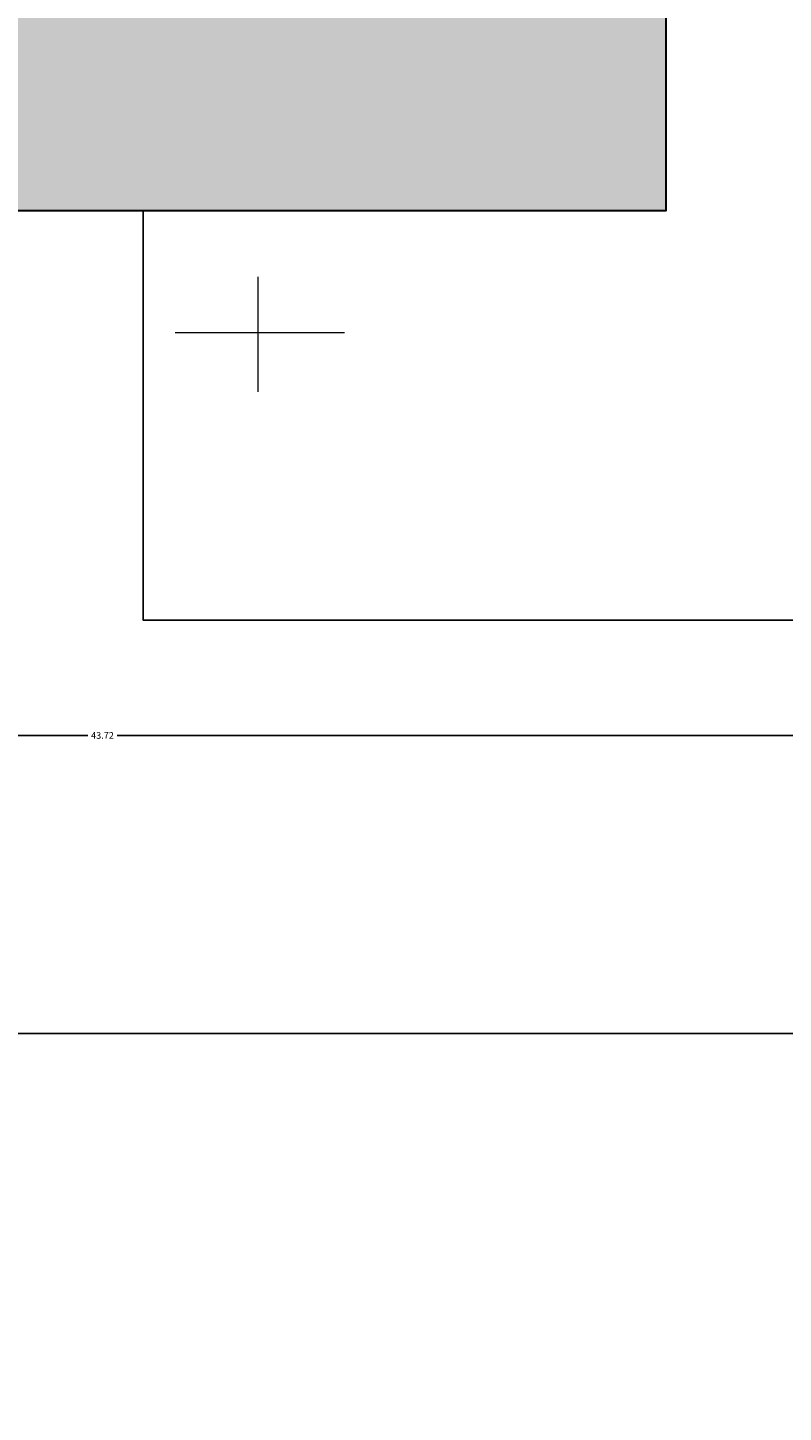
# Model space of a CAD drawing. Units: millimetres. Extents: x -8 to 285, y 5 to 221.
# Tile 12 of 30: x 27 to 47, y 113 to 150. Entities that reach past the tile are written whole.
import ezdxf

# ---------------------------------------------------------------- set-up
doc = ezdxf.new("R2010")
doc.units = ezdxf.units.MM
for name, color, linetype, lineweight in [('A-ANNO-DIMS', 2, 'Continuous', 18), ('E-ANNO-SYMB', 7, 'Continuous', 18), ('E-EQPM-PATT', 252, 'Continuous', 13), ('E-POWR-DC-LINK', 4, 'Continuous', 25), ('E-POWR-PV', 7, 'Continuous', 30)]:
    doc.layers.add(name, color=color, linetype=linetype, lineweight=lineweight)
doc.layers.add('E-POWR-DC-POS', color=30, linetype='Continuous', lineweight=25, true_color=0xf26722)
doc.styles.get("Standard").update_dxf_attribs({"font": 'arial.ttf'})
doc.dimstyles.get("Standard").update_dxf_attribs({"dimtxt": 0.18, "dimasz": 0.18, "dimexe": 0.18, "dimexo": 0.0625, "dimgap": 0.09, "dimtad": 0, "dimtih": 1, "dimtoh": 1, "dimdec": 4, "dimzin": 0, "dimdsep": 46, "dimtxsty": 'Standard', "dimcen": 0.09, "dimadec": 0, "dimazin": 0, "dimtfac": 1, "dimtdec": 4, "dimtofl": 0, "dimtmove": 0, "dimatfit": 3, "dimfxl": 1, "dimtolj": 1, "dimtzin": 0, "dimarcsym": 0})

# ---------------------------------------------------------------- blocks, each defined once
blk = doc.blocks.new('PV-MODULE-12V')
blk.add_lwpolyline([(0, 47), (37, 47), (37, 0), (0, 0)], close=True)
blk = doc.blocks.new('POLARITY-POSITIVE')
for p, q in [((2.22, 3.095), (2.22, 0)), ((0, 1.599), (4.543, 1.599))]:
    blk.add_line(p, q)
blk = doc.blocks.new('*D9')
at = {"layer": 'A-ANNO-DIMS', "color": 0, "lineweight": -2, "transparency": 16777216}
for p, q in [((6.672, 133.79), (6.672, 220.737)), ((270.919, 206.519), (270.919, 220.737)), ((6.852, 220.557), (138.33, 220.557)), ((270.739, 220.557), (139.262, 220.557))]:
    blk.add_line(p, q, dxfattribs=at)
at = {"layer": 'A-ANNO-DIMS', "color": 0, "transparency": 16777216}
for points in [[(6.852, 220.587), (6.852, 220.527), (6.672, 220.557)], [(270.739, 220.587), (270.739, 220.527), (270.919, 220.557)]]:
    blk.add_solid(points, dxfattribs=at)
at = {"layer": 'Defpoints', "color": 0, "transparency": 16777216}
for p in [(270.919, 220.557), (270.919, 206.457), (6.672, 133.727)]:
    blk.add_point(p, dxfattribs=at)
at = {"layer": 'A-ANNO-DIMS', "color": 0, "transparency": 16777216, "insert": (138.796, 220.557), "char_height": 0.18, "attachment_point": 5}
blk.add_mtext('\\A1;264.25', dxfattribs=at)
blk = doc.blocks.new('*D10')
at = {"layer": 'A-ANNO-DIMS', "color": 0, "lineweight": -2, "transparency": 16777216}
for p, q in [((145.103, 206.457), (-7.608, 206.457)), ((-7.428, 206.277), (-7.428, 113.161)), ((-7.428, 19.682), (-7.428, 112.797)), ((30.453, 19.502), (-7.608, 19.502))]:
    blk.add_line(p, q, dxfattribs=at)
at = {"layer": 'A-ANNO-DIMS', "color": 0, "transparency": 16777216}
for points in [[(-7.458, 206.277), (-7.398, 206.277), (-7.428, 206.457)], [(-7.458, 19.682), (-7.398, 19.682), (-7.428, 19.502)]]:
    blk.add_solid(points, dxfattribs=at)
at = {"layer": 'Defpoints', "color": 0, "transparency": 16777216}
for p in [(-7.428, 206.457), (145.165, 206.457), (30.516, 19.502)]:
    blk.add_point(p, dxfattribs=at)
at = {"layer": 'A-ANNO-DIMS', "color": 0, "transparency": 16777216, "insert": (-7.428, 112.979), "char_height": 0.18, "attachment_point": 5}
blk.add_mtext('\\A1;186.95', dxfattribs=at)
blk = doc.blocks.new('*D11')
at = {"layer": 'A-ANNO-DIMS', "color": 0, "lineweight": -2, "transparency": 16777216}
for p, q in [((6.853, 145.209), (6.853, 130.991)), ((50.572, 145.209), (50.572, 130.991)), ((7.033, 131.171), (28.316, 131.171)), ((50.392, 131.171), (29.109, 131.171))]:
    blk.add_line(p, q, dxfattribs=at)
at = {"layer": 'A-ANNO-DIMS', "color": 0, "transparency": 16777216}
for points in [[(7.033, 131.201), (7.033, 131.141), (6.853, 131.171)], [(50.392, 131.201), (50.392, 131.141), (50.572, 131.171)]]:
    blk.add_solid(points, dxfattribs=at)
at = {"layer": 'Defpoints', "color": 0, "transparency": 16777216}
for p in [(6.853, 145.271), (50.572, 145.271), (6.853, 131.171)]:
    blk.add_point(p, dxfattribs=at)
at = {"layer": 'A-ANNO-DIMS', "color": 0, "transparency": 16777216, "insert": (28.713, 131.171), "char_height": 0.18, "attachment_point": 5}
blk.add_mtext('\\A1;43.72', dxfattribs=at)

msp = doc.modelspace()

# ---------------------------------------------------------------- hatches: boundary and pattern name
at = {"layer": 'E-EQPM-PATT'}
h = msp.add_hatch(color=256, dxfattribs=at)
h.set_gradient(color2=(0, 0, 0), tint=1)
h.paths.add_polyline_path([(6.8535, 192.2715), (6.8535, 145.2715), (43.8535, 145.2715), (43.8535, 192.2715)])
h.paths.add_polyline_path([(37.8535, 186.2715), (37.8535, 151.2715), (12.8535, 151.2715), (12.8535, 186.2715)], flags=0)
h.paths.add_polyline_path([(50.5716, 145.2715), (87.5716, 145.2715), (87.5716, 192.2715), (50.5716, 192.2715)])
h.paths.add_polyline_path([(56.5716, 186.2715), (81.5716, 186.2715), (81.5716, 151.2715), (56.5716, 151.2715)], flags=0)
h.paths.add_polyline_path([(37.8535, 176.7715), (37.8535, 186.2715), (25.3535, 186.2715), (25.3535, 176.7715)], flags=0)
h.paths.add_polyline_path([(37.8535, 176.7715), (37.8535, 186.2715), (12.8535, 186.2715), (12.8535, 176.7715)], flags=0)
h.paths.add_polyline_path([(25.3535, 160.7715), (37.8535, 160.7715), (37.8535, 186.2715), (25.3535, 186.2715)], flags=0)
h.paths.add_polyline_path([(12.8535, 151.2715), (37.8535, 151.2715), (37.8535, 186.2715), (12.8535, 186.2715)], flags=16)
h.paths.add_polyline_path([(56.5716, 186.2715), (56.5716, 160.7715), (81.5716, 160.7715), (81.5716, 186.2715)], flags=0)
h.paths.add_polyline_path([(56.5716, 151.2715), (81.5716, 151.2715), (81.5716, 186.2715), (56.5716, 186.2715)], flags=16)

# ---------------------------------------------------------------- linework, layer by layer
at = {"layer": 'E-POWR-DC-LINK'}
msp.add_lwpolyline([(29.8062, 145.2715), (29.8062, 134.2715), (64.3247, 134.2715), (64.3247, 145.2715)], dxfattribs=at)
at = {"layer": 'E-POWR-DC-POS'}
msp.add_lwpolyline([(74.9801, 145.2715), (74.9801, 123.1618), (17.279, 123.1618), (17.279, 54.6776), (40.1717, 54.6776), (40.1717, 67.9064)], dxfattribs=at)

# ---------------------------------------------------------------- block references
at = {"layer": 'E-ANNO-SYMB'}
msp.add_blockref('POLARITY-POSITIVE', (30.6716, 140.4032), dxfattribs=at)
at = {"layer": 'E-POWR-PV'}
msp.add_blockref('PV-MODULE-12V', (6.853, 145.271), dxfattribs=at)

# ---------------------------------------------------------------- dimensions: what is measured, and where the dimension line sits
at = {"layer": 'A-ANNO-DIMS'}
dim = msp.add_linear_dim(base=(270.9192, 220.5568), p1=(6.6725, 133.7273), p2=(270.9192, 206.4568), dimstyle='Standard', override={"dimdec": 2, "dimlfac": 1, "dimrnd": 0, "dimzin": 0, "dimdsep": 46, "dimlunit": 2}, dxfattribs=at)
dim.commit()
dim.dimension.update_dxf_attribs({"geometry": '*D9', "text_midpoint": (138.7958, 220.5568)})
for base, p1, p2, angle, picture, middle in [((-7.4275, 206.4568), (30.516, 19.502), (145.1651, 206.4568), 90, '*D10', (-7.4275, 112.9794)), ((6.8535, 131.1715), (50.5716, 145.2715), (6.8535, 145.2715), 180, '*D11', (28.7125, 131.1715))]:
    dim = msp.add_linear_dim(base=base, p1=p1, p2=p2, angle=angle, dimstyle='Standard', override={"dimdec": 2, "dimlfac": 1, "dimrnd": 0, "dimzin": 0, "dimdsep": 46, "dimlunit": 2}, dxfattribs=at)
    dim.commit()
    dim.dimension.update_dxf_attribs({"geometry": picture, "text_midpoint": middle})

doc.saveas('drawing.dxf')
